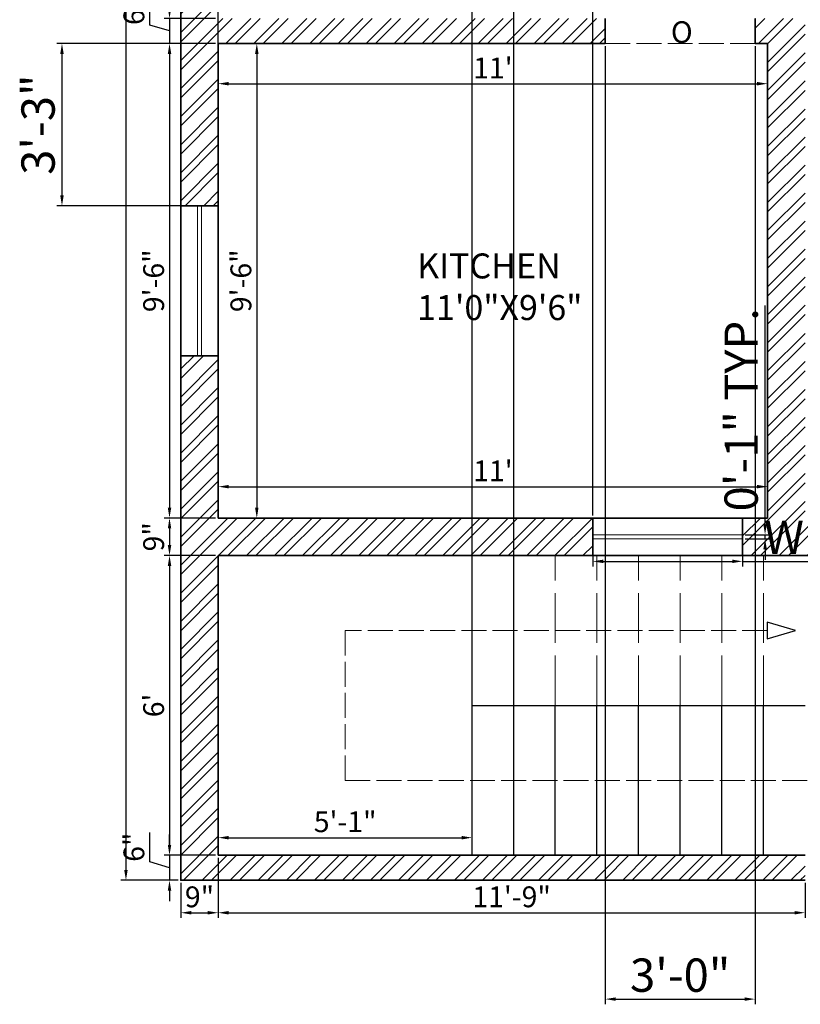
# Model space of a CAD drawing. Units: inches. Extents: x 3595 to 4516, y 2363 to 2965.
# Tile 1 of 12: x 3601 to 3789, y 2369 to 2606. Entities that reach past the tile are written whole.
import ezdxf

# ---------------------------------------------------------------- set-up
doc = ezdxf.new("R2010")
doc.units = ezdxf.units.IN
doc.linetypes.add('ACAD_ISO02W100', pattern=[15, 12, -3])
for name, color, linetype, lineweight in [('A-ANNO-DIMS', 2, 'Continuous', 18), ('A-ANNO-TEXT', 7, 'Continuous', 25), ('A-AREA-IDEN', 7, 'Continuous', 18), ('A-FLOR-STRS', 7, 'Continuous', 25), ('A-FLOR-STRS-OVHD', 7, 'ACAD_ISO02W100', 18), ('A-GLAZ', 4, 'Continuous', 18), ('A-WALL', 7, 'Continuous', 35), ('A-WALL-OVHD', 7, 'ACAD_ISO02W100', 18)]:
    doc.layers.add(name, color=color, linetype=linetype, lineweight=lineweight)
doc.layers.add('A-WALL-PATT', color=251, linetype='Continuous', lineweight=13, true_color=0x636466)
doc.styles.get("Standard").update_dxf_attribs({"font": 'arial.ttf'})
doc.dimstyles.new('ISO-25', dxfattribs={"dimtxt": 8, "dimasz": 2.5, "dimexe": 1.25, "dimexo": 0.625, "dimtad": 1, "dimdec": 1, "dimlunit": 3, "dimtxsty": 'Standard', "dimcen": 2.5, "dimadec": 0, "dimazin": 0, "dimtfac": 1, "dimtdec": 1, "dimtmove": 0, "dimatfit": 3, "dimfxl": 1, "dimarcsym": 0})

# ---------------------------------------------------------------- blocks, each defined once
blk = doc.blocks.new('*D48')
at = {"layer": 'A-ANNO-DIMS', "color": 0, "lineweight": -2, "transparency": 16777216}
for p, q in [((3649.52, 2600.04), (3659.41, 2600.04)), ((3658.16, 2597.54), (3658.16, 2488.54)), ((3649.52, 2486.04), (3659.41, 2486.04))]:
    blk.add_line(p, q, dxfattribs=at)
at = {"layer": 'A-ANNO-DIMS', "color": 0, "transparency": 16777216}
for points in [[(3657.74, 2597.54), (3658.57, 2597.54), (3658.16, 2600.04)], [(3657.74, 2488.54), (3658.57, 2488.54), (3658.16, 2486.04)]]:
    blk.add_solid(points, dxfattribs=at)
at = {"layer": 'Defpoints', "color": 0, "transparency": 16777216}
for p in [(3648.89, 2600.04), (3648.89, 2486.04), (3658.16, 2486.04)]:
    blk.add_point(p, dxfattribs=at)
at = {"layer": 'A-ANNO-DIMS', "color": 0, "transparency": 16777216, "insert": (3654.98, 2543.04), "char_height": 5, "attachment_point": 5, "rotation": 90}
blk.add_mtext('9\'-6"', dxfattribs=at)
blk = doc.blocks.new('*D49')
at = {"layer": 'A-ANNO-DIMS', "color": 0, "lineweight": -2, "transparency": 16777216}
for p, q in [((3648.89, 2599.42), (3648.89, 2589.13)), ((3780.89, 2599.42), (3780.89, 2589.13)), ((3651.39, 2590.38), (3778.39, 2590.38))]:
    blk.add_line(p, q, dxfattribs=at)
at = {"layer": 'A-ANNO-DIMS', "color": 0, "transparency": 16777216}
for points in [[(3651.39, 2590.79), (3651.39, 2589.96), (3648.89, 2590.38)], [(3778.39, 2590.79), (3778.39, 2589.96), (3780.89, 2590.38)]]:
    blk.add_solid(points, dxfattribs=at)
at = {"layer": 'Defpoints', "color": 0, "transparency": 16777216}
for p in [(3648.89, 2600.04), (3780.89, 2600.04), (3780.89, 2590.38)]:
    blk.add_point(p, dxfattribs=at)
at = {"layer": 'A-ANNO-DIMS', "color": 0, "transparency": 16777216, "insert": (3714.89, 2593.51), "char_height": 5, "attachment_point": 5}
blk.add_mtext("11'", dxfattribs=at)
blk = doc.blocks.new('*D55')
at = {"layer": 'A-ANNO-DIMS', "color": 0, "lineweight": -2, "transparency": 16777216}
for p, q in [((3648.89, 2486.67), (3648.89, 2494.83)), ((3651.39, 2493.58), (3778.39, 2493.58)), ((3780.89, 2486.67), (3780.89, 2494.83))]:
    blk.add_line(p, q, dxfattribs=at)
at = {"layer": 'A-ANNO-DIMS', "color": 0, "transparency": 16777216}
for points in [[(3651.39, 2494), (3651.39, 2493.17), (3648.89, 2493.58)], [(3778.39, 2494), (3778.39, 2493.17), (3780.89, 2493.58)]]:
    blk.add_solid(points, dxfattribs=at)
at = {"layer": 'Defpoints', "color": 0, "transparency": 16777216}
for p in [(3780.89, 2493.58), (3648.89, 2486.04), (3780.89, 2486.04)]:
    blk.add_point(p, dxfattribs=at)
at = {"layer": 'A-ANNO-DIMS', "color": 0, "transparency": 16777216, "insert": (3714.89, 2496.72), "char_height": 5, "attachment_point": 5}
blk.add_mtext("11'", dxfattribs=at)
blk = doc.blocks.new('*D56')
at = {"layer": 'A-ANNO-DIMS', "color": 0, "lineweight": -2, "transparency": 16777216}
for p, q in [((3648.89, 2405.67), (3648.89, 2410.52)), ((3709.89, 2405.67), (3709.89, 2410.52)), ((3651.39, 2409.27), (3707.39, 2409.27))]:
    blk.add_line(p, q, dxfattribs=at)
at = {"layer": 'A-ANNO-DIMS', "color": 0, "transparency": 16777216}
for points in [[(3651.39, 2409.69), (3651.39, 2408.85), (3648.89, 2409.27)], [(3707.39, 2409.69), (3707.39, 2408.85), (3709.89, 2409.27)]]:
    blk.add_solid(points, dxfattribs=at)
at = {"layer": 'Defpoints', "color": 0, "transparency": 16777216}
for p in [(3709.89, 2409.27), (3648.89, 2405.04), (3709.89, 2405.04)]:
    blk.add_point(p, dxfattribs=at)
at = {"layer": 'A-ANNO-DIMS', "color": 0, "transparency": 16777216, "insert": (3679.39, 2412.45), "char_height": 5, "attachment_point": 5}
blk.add_mtext('5\'-1"', dxfattribs=at)
blk = doc.blocks.new('*D73')
at = {"layer": 'A-ANNO-DIMS', "color": 0, "lineweight": -2, "transparency": 16777216}
for p, q in [((3632.44, 2604.47), (3632.44, 2611.49)), ((3637.18, 2608.54), (3637.18, 2611.04)), ((3637.18, 2603.04), (3632.44, 2604.47)), ((3648.27, 2606.04), (3635.93, 2606.04)), ((3637.18, 2606.04), (3637.18, 2600.04)), ((3637.18, 2606.04), (3637.18, 2600.04)), ((3648.27, 2600.04), (3635.93, 2600.04)), ((3637.18, 2597.54), (3637.18, 2595.04))]:
    blk.add_line(p, q, dxfattribs=at)
at = {"layer": 'A-ANNO-DIMS', "color": 0, "transparency": 16777216}
for points in [[(3636.77, 2608.54), (3637.6, 2608.54), (3637.18, 2606.04)], [(3636.77, 2597.54), (3637.6, 2597.54), (3637.18, 2600.04)]]:
    blk.add_solid(points, dxfattribs=at)
at = {"layer": 'Defpoints', "color": 0, "transparency": 16777216}
for p in [(3648.89, 2606.04), (3637.18, 2600.04), (3648.89, 2600.04)]:
    blk.add_point(p, dxfattribs=at)
at = {"layer": 'A-ANNO-DIMS', "color": 0, "transparency": 16777216, "insert": (3629.27, 2607.98), "char_height": 5, "attachment_point": 5, "rotation": 90}
blk.add_mtext('6"', dxfattribs=at)
blk = doc.blocks.new('*D74')
at = {"layer": 'A-ANNO-DIMS', "color": 0, "lineweight": -2, "transparency": 16777216}
for p, q in [((3648.27, 2600.04), (3635.93, 2600.04)), ((3637.18, 2597.54), (3637.18, 2488.54)), ((3648.27, 2486.04), (3635.93, 2486.04))]:
    blk.add_line(p, q, dxfattribs=at)
at = {"layer": 'A-ANNO-DIMS', "color": 0, "transparency": 16777216}
for points in [[(3636.77, 2597.54), (3637.6, 2597.54), (3637.18, 2600.04)], [(3636.77, 2488.54), (3637.6, 2488.54), (3637.18, 2486.04)]]:
    blk.add_solid(points, dxfattribs=at)
at = {"layer": 'Defpoints', "color": 0, "transparency": 16777216}
for p in [(3648.89, 2600.04), (3637.18, 2486.04), (3648.89, 2486.04)]:
    blk.add_point(p, dxfattribs=at)
at = {"layer": 'A-ANNO-DIMS', "color": 0, "transparency": 16777216, "insert": (3634.01, 2543.04), "char_height": 5, "attachment_point": 5, "rotation": 90}
blk.add_mtext('9\'-6"', dxfattribs=at)
blk = doc.blocks.new('*D75')
at = {"layer": 'A-ANNO-DIMS', "color": 0, "lineweight": -2, "transparency": 16777216}
for p, q in [((3648.27, 2486.04), (3635.93, 2486.04)), ((3637.18, 2483.54), (3637.18, 2479.54)), ((3648.27, 2477.04), (3635.93, 2477.04))]:
    blk.add_line(p, q, dxfattribs=at)
at = {"layer": 'A-ANNO-DIMS', "color": 0, "transparency": 16777216}
for points in [[(3636.77, 2483.54), (3637.6, 2483.54), (3637.18, 2486.04)], [(3636.77, 2479.54), (3637.6, 2479.54), (3637.18, 2477.04)]]:
    blk.add_solid(points, dxfattribs=at)
at = {"layer": 'Defpoints', "color": 0, "transparency": 16777216}
for p in [(3648.89, 2486.04), (3637.18, 2477.04), (3648.89, 2477.04)]:
    blk.add_point(p, dxfattribs=at)
at = {"layer": 'A-ANNO-DIMS', "color": 0, "transparency": 16777216, "insert": (3634.01, 2481.54), "char_height": 5, "attachment_point": 5, "rotation": 90}
blk.add_mtext('9"', dxfattribs=at)
blk = doc.blocks.new('*D76')
at = {"layer": 'A-ANNO-DIMS', "color": 0, "lineweight": -2, "transparency": 16777216}
for p, q in [((3648.27, 2477.04), (3635.93, 2477.04)), ((3637.18, 2474.54), (3637.18, 2407.54)), ((3648.27, 2405.04), (3635.93, 2405.04))]:
    blk.add_line(p, q, dxfattribs=at)
at = {"layer": 'A-ANNO-DIMS', "color": 0, "transparency": 16777216}
for points in [[(3636.77, 2474.54), (3637.6, 2474.54), (3637.18, 2477.04)], [(3636.77, 2407.54), (3637.6, 2407.54), (3637.18, 2405.04)]]:
    blk.add_solid(points, dxfattribs=at)
at = {"layer": 'Defpoints', "color": 0, "transparency": 16777216}
for p in [(3648.89, 2477.04), (3637.18, 2405.04), (3648.89, 2405.04)]:
    blk.add_point(p, dxfattribs=at)
at = {"layer": 'A-ANNO-DIMS', "color": 0, "transparency": 16777216, "insert": (3634.01, 2441.04), "char_height": 5, "attachment_point": 5, "rotation": 90}
blk.add_mtext("6'", dxfattribs=at)
blk = doc.blocks.new('*D77')
at = {"layer": 'A-ANNO-DIMS', "color": 0, "lineweight": -2, "transparency": 16777216}
for p, q in [((3632.44, 2403.47), (3632.44, 2410.49)), ((3637.18, 2407.54), (3637.18, 2410.04)), ((3637.18, 2402.04), (3632.44, 2403.47)), ((3648.27, 2405.04), (3635.93, 2405.04)), ((3637.18, 2405.04), (3637.18, 2399.04)), ((3637.18, 2405.04), (3637.18, 2399.04)), ((3639.27, 2399.04), (3635.93, 2399.04)), ((3637.18, 2396.54), (3637.18, 2394.04))]:
    blk.add_line(p, q, dxfattribs=at)
at = {"layer": 'A-ANNO-DIMS', "color": 0, "transparency": 16777216}
for points in [[(3636.77, 2407.54), (3637.6, 2407.54), (3637.18, 2405.04)], [(3636.77, 2396.54), (3637.6, 2396.54), (3637.18, 2399.04)]]:
    blk.add_solid(points, dxfattribs=at)
at = {"layer": 'Defpoints', "color": 0, "transparency": 16777216}
for p in [(3648.89, 2405.04), (3637.18, 2399.04), (3639.89, 2399.04)]:
    blk.add_point(p, dxfattribs=at)
at = {"layer": 'A-ANNO-DIMS', "color": 0, "transparency": 16777216, "insert": (3629.27, 2406.98), "char_height": 5, "attachment_point": 5, "rotation": 90}
blk.add_mtext('6"', dxfattribs=at)
blk = doc.blocks.new('*D78')
at = {"layer": 'A-ANNO-DIMS', "color": 0, "lineweight": -2, "transparency": 16777216}
for p, q in [((3648.89, 2404.42), (3648.89, 2389.99)), ((3639.89, 2398.42), (3639.89, 2389.99)), ((3642.39, 2391.24), (3646.39, 2391.24))]:
    blk.add_line(p, q, dxfattribs=at)
at = {"layer": 'A-ANNO-DIMS', "color": 0, "transparency": 16777216}
for points in [[(3642.39, 2391.65), (3642.39, 2390.82), (3639.89, 2391.24)], [(3646.39, 2391.65), (3646.39, 2390.82), (3648.89, 2391.24)]]:
    blk.add_solid(points, dxfattribs=at)
at = {"layer": 'Defpoints', "color": 0, "transparency": 16777216}
for p in [(3648.89, 2405.04), (3639.89, 2399.04), (3648.89, 2391.24)]:
    blk.add_point(p, dxfattribs=at)
at = {"layer": 'A-ANNO-DIMS', "color": 0, "transparency": 16777216, "insert": (3644.39, 2394.41), "char_height": 5, "attachment_point": 5}
blk.add_mtext('9"', dxfattribs=at)
blk = doc.blocks.new('*D79')
at = {"layer": 'A-ANNO-DIMS', "color": 0, "lineweight": -2, "transparency": 16777216}
for p, q in [((3648.89, 2404.42), (3648.89, 2389.99)), ((3789.89, 2398.42), (3789.89, 2389.99)), ((3651.39, 2391.24), (3787.39, 2391.24))]:
    blk.add_line(p, q, dxfattribs=at)
at = {"layer": 'A-ANNO-DIMS', "color": 0, "transparency": 16777216}
for points in [[(3651.39, 2391.65), (3651.39, 2390.82), (3648.89, 2391.24)], [(3787.39, 2391.65), (3787.39, 2390.82), (3789.89, 2391.24)]]:
    blk.add_solid(points, dxfattribs=at)
at = {"layer": 'Defpoints', "color": 0, "transparency": 16777216}
for p in [(3648.89, 2405.04), (3789.89, 2399.04), (3789.89, 2391.24)]:
    blk.add_point(p, dxfattribs=at)
at = {"layer": 'A-ANNO-DIMS', "color": 0, "transparency": 16777216, "insert": (3719.39, 2394.41), "char_height": 5, "attachment_point": 5}
blk.add_mtext('11\'-9"', dxfattribs=at)
blk = doc.blocks.new('*D90')
at = {"layer": 'A-ANNO-DIMS', "color": 0, "lineweight": -2, "transparency": 16777216}
for p, q in [((3639.27, 2903.04), (3625.46, 2903.04)), ((3626.71, 2900.54), (3626.71, 2401.54)), ((3639.27, 2399.04), (3625.46, 2399.04))]:
    blk.add_line(p, q, dxfattribs=at)
at = {"layer": 'A-ANNO-DIMS', "color": 0, "transparency": 16777216}
for points in [[(3626.3, 2900.54), (3627.13, 2900.54), (3626.71, 2903.04)], [(3626.3, 2401.54), (3627.13, 2401.54), (3626.71, 2399.04)]]:
    blk.add_solid(points, dxfattribs=at)
at = {"layer": 'Defpoints', "color": 0, "transparency": 16777216}
for p in [(3639.89, 2903.04), (3626.71, 2399.04), (3639.89, 2399.04)]:
    blk.add_point(p, dxfattribs=at)
at = {"layer": 'A-ANNO-DIMS', "color": 0, "transparency": 16777216, "insert": (3623.58, 2651.04), "char_height": 5, "attachment_point": 5, "rotation": 90}
blk.add_mtext("42'", dxfattribs=at)
blk = doc.blocks.new('WIN-GLAZING-36IN')
for p, q in [((0, 1), (36, 1)), ((0, 0), (36, 0))]:
    blk.add_line(p, q)
blk = doc.blocks.new('*D101')
at = {"layer": 'A-ANNO-DIMS', "color": 0, "lineweight": -2, "transparency": 16777216}
for p, q in [((3738.89, 2480.42), (3738.89, 2474.39)), ((3774.89, 2480.42), (3774.89, 2474.39)), ((3741.39, 2475.64), (3772.39, 2475.64)), ((3774.89, 2475.64), (3879.88, 2475.64))]:
    blk.add_line(p, q, dxfattribs=at)
at = {"layer": 'A-ANNO-DIMS', "color": 0, "transparency": 16777216}
for points in [[(3741.39, 2476.06), (3741.39, 2475.23), (3738.89, 2475.64)], [(3772.39, 2476.06), (3772.39, 2475.23), (3774.89, 2475.64)]]:
    blk.add_solid(points, dxfattribs=at)
at = {"layer": 'Defpoints', "color": 0, "transparency": 16777216}
for p in [(3738.89, 2481.04), (3774.89, 2481.04), (3774.89, 2475.64)]:
    blk.add_point(p, dxfattribs=at)
at = {"layer": 'A-ANNO-DIMS', "color": 0, "transparency": 16777216, "insert": (3828.63, 2480.41), "char_height": 8, "attachment_point": 5}
blk.add_mtext('WINDOW 3\'-0" TYP.', dxfattribs=at)
blk = doc.blocks.new('*D102')
at = {"layer": 'A-ANNO-DIMS', "color": 0, "lineweight": -2, "transparency": 16777216}
for p, q in [((3780.29, 2484.54), (3780.29, 2537.06)), ((3775.52, 2482.04), (3781.54, 2482.04)), ((3775.52, 2481.04), (3781.54, 2481.04)), ((3780.29, 2481.04), (3780.29, 2482.04)), ((3780.29, 2478.54), (3780.29, 2476.04))]:
    blk.add_line(p, q, dxfattribs=at)
at = {"layer": 'A-ANNO-DIMS', "color": 0, "transparency": 16777216}
for points in [[(3779.88, 2484.54), (3780.71, 2484.54), (3780.29, 2482.04)], [(3779.88, 2478.54), (3780.71, 2478.54), (3780.29, 2481.04)]]:
    blk.add_solid(points, dxfattribs=at)
at = {"layer": 'Defpoints', "color": 0, "transparency": 16777216}
for p in [(3774.89, 2482.04), (3774.89, 2481.04), (3780.29, 2482.04)]:
    blk.add_point(p, dxfattribs=at)
at = {"layer": 'A-ANNO-DIMS', "color": 0, "transparency": 16777216, "insert": (3775.58, 2512.05), "char_height": 8, "attachment_point": 5, "rotation": 90}
blk.add_mtext('0\'-1" TYP.', dxfattribs=at)
blk = doc.blocks.new('*D152')
at = {"layer": 'A-ANNO-DIMS', "color": 0, "lineweight": -2, "transparency": 16777216}
for p, q in [((3648.27, 2600.04), (3610.09, 2600.04)), ((3611.34, 2597.54), (3611.34, 2563.54)), ((3648.27, 2561.04), (3610.09, 2561.04))]:
    blk.add_line(p, q, dxfattribs=at)
at = {"layer": 'A-ANNO-DIMS', "color": 0, "transparency": 16777216}
for points in [[(3610.93, 2597.54), (3611.76, 2597.54), (3611.34, 2600.04)], [(3610.93, 2563.54), (3611.76, 2563.54), (3611.34, 2561.04)]]:
    blk.add_solid(points, dxfattribs=at)
at = {"layer": 'Defpoints', "color": 0, "transparency": 16777216}
for p in [(3648.89, 2600.04), (3611.34, 2561.04), (3648.89, 2561.04)]:
    blk.add_point(p, dxfattribs=at)
at = {"layer": 'A-ANNO-DIMS', "color": 0, "transparency": 16777216, "insert": (3606.63, 2580.54), "char_height": 8, "attachment_point": 5, "rotation": 90}
blk.add_mtext('3\'-3"', dxfattribs=at)
blk = doc.blocks.new('*D156')
at = {"layer": 'A-ANNO-DIMS', "color": 0, "lineweight": -2, "transparency": 16777216}
for p, q in [((3648.89, 2486.67), (3648.89, 2932.84)), ((3738.89, 2486.67), (3738.89, 2932.84)), ((3651.39, 2931.59), (3736.39, 2931.59))]:
    blk.add_line(p, q, dxfattribs=at)
at = {"layer": 'A-ANNO-DIMS', "color": 0, "transparency": 16777216}
for points in [[(3651.39, 2932.01), (3651.39, 2931.18), (3648.89, 2931.59)], [(3736.39, 2932.01), (3736.39, 2931.18), (3738.89, 2931.59)]]:
    blk.add_solid(points, dxfattribs=at)
at = {"layer": 'Defpoints', "color": 0, "transparency": 16777216}
for p in [(3738.89, 2931.59), (3648.89, 2486.04), (3738.89, 2486.04)]:
    blk.add_point(p, dxfattribs=at)
at = {"layer": 'A-ANNO-DIMS', "color": 0, "transparency": 16777216, "insert": (3693.89, 2936.3), "char_height": 8, "attachment_point": 5}
blk.add_mtext('7\'-6"', dxfattribs=at)
blk = doc.blocks.new('*D158')
at = {"layer": 'A-ANNO-DIMS', "color": 0, "lineweight": -2, "transparency": 16777216}
for p, q in [((3741.89, 2599.42), (3741.89, 2369.24)), ((3777.89, 2599.42), (3777.89, 2369.24)), ((3744.39, 2370.49), (3775.39, 2370.49))]:
    blk.add_line(p, q, dxfattribs=at)
at = {"layer": 'A-ANNO-DIMS', "color": 0, "transparency": 16777216}
for points in [[(3744.39, 2370.91), (3744.39, 2370.08), (3741.89, 2370.49)], [(3775.39, 2370.91), (3775.39, 2370.08), (3777.89, 2370.49)]]:
    blk.add_solid(points, dxfattribs=at)
at = {"layer": 'Defpoints', "color": 0, "transparency": 16777216}
for p in [(3741.89, 2600.04), (3777.89, 2600.04), (3777.89, 2370.49)]:
    blk.add_point(p, dxfattribs=at)
at = {"layer": 'A-ANNO-DIMS', "color": 0, "transparency": 16777216, "insert": (3759.89, 2375.21), "char_height": 8, "attachment_point": 5}
blk.add_mtext('3\'-0"', dxfattribs=at)
blk = doc.blocks.new('*D159')
at = {"layer": 'A-ANNO-DIMS', "color": 0, "lineweight": -2, "transparency": 16777216}
for p, q in [((3709.89, 2405.67), (3709.89, 2932.84)), ((3719.89, 2405.67), (3719.89, 2932.84)), ((3712.39, 2931.59), (3717.39, 2931.59)), ((3719.89, 2931.59), (3751.12, 2931.59))]:
    blk.add_line(p, q, dxfattribs=at)
at = {"layer": 'A-ANNO-DIMS', "color": 0, "transparency": 16777216}
for points in [[(3712.39, 2932.01), (3712.39, 2931.18), (3709.89, 2931.59)], [(3717.39, 2932.01), (3717.39, 2931.18), (3719.89, 2931.59)]]:
    blk.add_solid(points, dxfattribs=at)
at = {"layer": 'Defpoints', "color": 0, "transparency": 16777216}
for p in [(3719.89, 2931.59), (3709.89, 2405.04), (3719.89, 2405.04)]:
    blk.add_point(p, dxfattribs=at)
at = {"layer": 'A-ANNO-DIMS', "color": 0, "transparency": 16777216, "insert": (3736.76, 2936.3), "char_height": 8, "attachment_point": 5}
blk.add_mtext('0\'-10"', dxfattribs=at)

msp = doc.modelspace()

# ---------------------------------------------------------------- hatches: boundary and pattern name
at = {"layer": 'A-WALL-PATT'}
h = msp.add_hatch(dxfattribs=at)
h.set_pattern_fill('ANSI32', color=256, scale=0.5)
h.paths.add_polyline_path([(3648.89, 2894.04), (3726.89, 2894.04), (3726.89, 2903.04), (3639.89, 2903.04), (3639.89, 2756.04), (3648.89, 2756.04)])
h.paths.add_polyline_path([(3800.39, 2903.04), (3774.89, 2903.04), (3774.89, 2894.04), (3780.89, 2894.04), (3780.89, 2792.04), (3789.89, 2792.04), (3789.89, 2894.04), (3800.39, 2894.04)])
h.paths.add_polyline_path([(3882.89, 2903.04), (3836.39, 2903.04), (3836.39, 2894.04), (3846.89, 2894.04), (3846.89, 2798.04), (3819.89, 2798.04), (3819.89, 2792.04), (3846.89, 2792.04), (3846.89, 2756.04), (3780.89, 2756.04), (3780.89, 2702.04), (3777.89, 2702.04), (3777.89, 2693.04), (3800.39, 2693.04), (3800.39, 2702.04), (3789.89, 2702.04), (3789.89, 2750.04), (3846.89, 2750.04), (3846.89, 2702.04), (3836.39, 2702.04), (3836.39, 2693.04), (3951.89, 2693.04), (3951.89, 2702.04), (3852.89, 2702.04), (3852.89, 2840.04), (3954.89, 2840.04), (3954.89, 2846.04), (3852.89, 2846.04), (3852.89, 2894.04), (3882.89, 2894.04)])
h.paths.add_polyline_path([(3999.89, 2903.04), (3918.89, 2903.04), (3918.89, 2894.04), (3948.89, 2894.04), (3948.89, 2876.04), (3954.89, 2876.04), (3954.89, 2894.04), (3990.89, 2894.04), (3990.89, 2795.04), (3999.89, 2795.04)])
h.paths.add_polyline_path([(3741.89, 2702.04), (3648.89, 2702.04), (3648.89, 2708.04), (3639.89, 2708.04), (3639.89, 2673.54), (3648.89, 2673.54), (3648.89, 2693.04), (3741.89, 2693.04)])
h.paths.add_polyline_path([(3648.89, 2600.04), (3741.89, 2600.04), (3741.89, 2606.04), (3648.89, 2606.04), (3648.89, 2625.54), (3639.89, 2625.54), (3639.89, 2561.04), (3648.89, 2561.04)])
h.paths.add_polyline_path([(3648.89, 2525.04), (3639.89, 2525.04), (3639.89, 2399.04), (3789.89, 2399.04), (3789.89, 2405.04), (3648.89, 2405.04), (3648.89, 2477.04), (3738.89, 2477.04), (3738.89, 2486.04), (3648.89, 2486.04)])
h.paths.add_polyline_path([(3789.89, 2606.04), (3777.89, 2606.04), (3777.89, 2600.04), (3780.89, 2600.04), (3780.89, 2486.04), (3774.89, 2486.04), (3774.89, 2477.04), (3831.89, 2477.04), (3831.89, 2486.04), (3789.89, 2486.04)])
h.paths.add_polyline_path([(3939.89, 2486.04), (3897.89, 2486.04), (3897.89, 2477.04), (3939.89, 2477.04)])
h.paths.add_polyline_path([(3999.89, 2511.54), (3990.89, 2511.54), (3990.89, 2486.04), (3987.89, 2486.04), (3987.89, 2477.04), (3999.89, 2477.04)])
h.paths.add_polyline_path([(3999.89, 2607.54), (3990.89, 2607.54), (3990.89, 2571.54), (3999.89, 2571.54)])
h.paths.add_polyline_path([(3999.89, 2747.04), (3990.89, 2747.04), (3990.89, 2702.04), (3987.89, 2702.04), (3987.89, 2693.04), (3990.89, 2693.04), (3990.89, 2667.54), (3999.89, 2667.54)])

# ---------------------------------------------------------------- linework, layer by layer
at = {"layer": 'A-FLOR-STRS'}
for p, q in [((3709.89, 2405.04), (3709.89, 2441.04)), ((3709.89, 2441.04), (3789.89, 2441.04)), ((3719.89, 2405.04), (3719.89, 2441.04)), ((3729.89, 2405.04), (3729.89, 2441.04)), ((3739.89, 2405.04), (3739.89, 2441.04)), ((3749.89, 2405.04), (3749.89, 2441.04)), ((3759.89, 2405.04), (3759.89, 2441.04)), ((3769.89, 2405.04), (3769.89, 2441.04)), ((3779.89, 2405.04), (3779.89, 2441.04))]:
    msp.add_line(p, q, dxfattribs=at)
msp.add_lwpolyline([(3787.63, 2459.04), (3780.82, 2461.04), (3780.82, 2457.04)], close=True, dxfattribs=at)
at = {"layer": 'A-FLOR-STRS-OVHD'}
for p, q in [((3709.89, 2441.04), (3709.89, 2477.04)), ((3719.89, 2441.04), (3719.89, 2477.04)), ((3729.89, 2441.04), (3729.89, 2477.04)), ((3739.89, 2441.04), (3739.89, 2477.04)), ((3749.89, 2441.04), (3749.89, 2477.04)), ((3759.89, 2441.04), (3759.89, 2477.04)), ((3769.89, 2441.04), (3769.89, 2477.04)), ((3779.89, 2441.04), (3779.89, 2477.04))]:
    msp.add_line(p, q, dxfattribs=at)
at = {"layer": 'A-FLOR-STRS-OVHD', "ltscale": 0.5}
msp.add_lwpolyline([(3780.82, 2459.04), (3679.39, 2459.04), (3679.39, 2423.04), (3798.62, 2423.04)], dxfattribs=at)
at = {"layer": 'A-WALL'}
for p, q in [((3741.89, 2606.04), (3741.89, 2600.04)), ((3777.89, 2606.04), (3777.89, 2600.04)), ((3648.89, 2600.04), (3741.89, 2600.04)), ((3648.89, 2486.04), (3648.89, 2600.04)), ((3777.89, 2600.04), (3780.89, 2600.04)), ((3780.89, 2486.04), (3780.89, 2600.04)), ((3648.89, 2561.04), (3639.89, 2561.04)), ((3648.89, 2525.04), (3639.89, 2525.04)), ((3648.89, 2486.04), (3780.89, 2486.04)), ((3738.89, 2477.04), (3738.89, 2486.04)), ((3774.89, 2477.04), (3774.89, 2486.04)), ((3648.89, 2405.04), (3648.89, 2477.04)), ((3648.89, 2477.04), (3939.89, 2477.04)), ((3648.89, 2405.04), (3789.89, 2405.04))]:
    msp.add_line(p, q, dxfattribs=at)
msp.add_lwpolyline([(3789.89, 2399.04), (3639.89, 2399.04), (3639.89, 2903.04), (3999.89, 2903.04), (3999.89, 2477.04)], dxfattribs=at)
at = {"layer": 'A-WALL-OVHD', "ltscale": 0.5}
msp.add_line((3741.89, 2600.04), (3777.89, 2600.04), dxfattribs=at)

# ---------------------------------------------------------------- block references
at = {"layer": 'A-GLAZ', "rotation": 269.9999999999999}
msp.add_blockref('WIN-GLAZING-36IN', (3643.89, 2561.04), dxfattribs=at)
at = {"layer": 'A-GLAZ'}
msp.add_blockref('WIN-GLAZING-36IN', (3738.89, 2481.04), dxfattribs=at)

# ---------------------------------------------------------------- texts
at = {"layer": 'A-ANNO-TEXT'}
msp.add_text('O', height=5.18, dxfattribs=at).set_placement((3757.66, 2600.18))
at = {"layer": 'A-AREA-IDEN', "insert": (3696.68, 2549.6), "char_height": 6, "attachment_point": 1}
msp.add_mtext_dynamic_manual_height_columns('{\\fTimes New Roman|b0|i0|c0|p18;KITCHEN\\P11\'0"X9\'6"}', width=67.3508, gutter_width=12.5, heights=[0], dxfattribs=at)

# ---------------------------------------------------------------- dimensions: what is measured, and where the dimension line sits
at = {"layer": 'A-ANNO-DIMS'}
for base, p1, p2, override, picture, middle in [((3738.89, 2931.59), (3648.89, 2486.04), (3738.89, 2486.04), {"dimdec": 1, "dimlfac": 1, "dimrnd": 0, "dimzin": 1, "dimdsep": 46, "dimlunit": 4, "dimfrac": 2}, '*D156', (3693.89, 2936.3)), ((3719.89, 2931.59), (3709.89, 2405.04), (3719.89, 2405.04), {"dimdec": 1, "dimlfac": 1, "dimrnd": 0, "dimzin": 1, "dimdsep": 46, "dimlunit": 4, "dimfrac": 2}, '*D159', (3736.76, 2936.3)), ((3780.89, 2590.38), (3648.89, 2600.04), (3780.89, 2600.04), {"dimtxt": 5, "dimclrd": 0, "dimclre": 0, "dimclrt": 0}, '*D49', (3714.89, 2593.51)), ((3777.89, 2370.49), (3741.89, 2600.04), (3777.89, 2600.04), {"dimdec": 1, "dimlfac": 1, "dimrnd": 0, "dimzin": 1, "dimdsep": 46, "dimlunit": 4, "dimfrac": 2}, '*D158', (3759.89, 2375.21)), ((3780.89, 2493.58), (3648.89, 2486.04), (3780.89, 2486.04), {"dimtxt": 5, "dimclrd": 0, "dimclre": 0, "dimclrt": 0}, '*D55', (3714.89, 2496.72)), ((3709.89, 2409.27), (3648.89, 2405.04), (3709.89, 2405.04), {"dimtxt": 5, "dimclrd": 0, "dimclre": 0, "dimclrt": 0}, '*D56', (3679.39, 2412.45)), ((3648.89, 2391.24), (3639.89, 2399.04), (3648.89, 2405.04), {"dimtxt": 5, "dimclrd": 0, "dimclre": 0, "dimclrt": 0}, '*D78', (3644.39, 2394.41)), ((3789.89, 2391.24), (3648.89, 2405.04), (3789.89, 2399.04), {"dimtxt": 5, "dimclrd": 0, "dimclre": 0, "dimclrt": 0, "dimtmove": 1}, '*D79', (3719.39, 2394.41))]:
    dim = msp.add_linear_dim(base=base, p1=p1, p2=p2, dimstyle='ISO-25', override=override, dxfattribs=at)
    dim.commit()
    dim.dimension.update_dxf_attribs({"geometry": picture, "text_midpoint": middle})
for base, p1, p2, override, picture, middle in [((3626.71, 2399.04), (3639.89, 2903.04), (3639.89, 2399.04), {"dimtxt": 5, "dimclrd": 0, "dimclre": 0, "dimclrt": 0}, '*D90', (3623.58, 2651.04)), ((3637.18, 2600.04), (3648.89, 2606.04), (3648.89, 2600.04), {"dimtxt": 5, "dimclrd": 0, "dimclre": 0, "dimclrt": 0, "dimtmove": 1}, '*D73', (3629.27, 2605.09)), ((3611.34, 2561.04), (3648.89, 2600.04), (3648.89, 2561.04), {"dimdec": 1, "dimlfac": 1, "dimrnd": 0, "dimzin": 1, "dimdsep": 46, "dimlunit": 4, "dimfrac": 2}, '*D152', (3606.63, 2580.54)), ((3637.18, 2486.04), (3648.89, 2600.04), (3648.89, 2486.04), {"dimtxt": 5, "dimclrd": 0, "dimclre": 0, "dimclrt": 0, "dimtmove": 1}, '*D74', (3634.01, 2543.04)), ((3658.16, 2486.04), (3648.89, 2600.04), (3648.89, 2486.04), {"dimtxt": 5, "dimclrd": 0, "dimclre": 0, "dimclrt": 0}, '*D48', (3654.98, 2543.04)), ((3637.18, 2477.04), (3648.89, 2486.04), (3648.89, 2477.04), {"dimtxt": 5, "dimclrd": 0, "dimclre": 0, "dimclrt": 0, "dimtmove": 1}, '*D75', (3634.01, 2481.54)), ((3637.18, 2405.04), (3648.89, 2477.04), (3648.89, 2405.04), {"dimtxt": 5, "dimclrd": 0, "dimclre": 0, "dimclrt": 0, "dimtmove": 1}, '*D76', (3634.01, 2441.04)), ((3637.18, 2399.04), (3648.89, 2405.04), (3639.89, 2399.04), {"dimtxt": 5, "dimclrd": 0, "dimclre": 0, "dimclrt": 0, "dimtmove": 1}, '*D77', (3629.27, 2404.09))]:
    dim = msp.add_linear_dim(base=base, p1=p1, p2=p2, angle=90, dimstyle='ISO-25', override=override, dxfattribs=at)
    dim.commit()
    dim.dimension.update_dxf_attribs({"geometry": picture, "text_midpoint": middle})
dim = msp.add_linear_dim(base=(3780.29, 2482.04), p1=(3774.89, 2481.04), p2=(3774.89, 2482.04), angle=90, text='<> TYP.', dimstyle='ISO-25', override={"dimdec": 1, "dimlfac": 1, "dimrnd": 0, "dimzin": 1, "dimdsep": 46, "dimlunit": 4, "dimfrac": 2}, dxfattribs=at)
dim.commit()
dim.dimension.update_dxf_attribs({"geometry": '*D102', "text_midpoint": (3775.58, 2512.05)})
dim = msp.add_linear_dim(base=(3774.89, 2475.64), p1=(3738.89, 2481.04), p2=(3774.89, 2481.04), text='WINDOW <> TYP.', dimstyle='ISO-25', override={"dimdec": 1, "dimlfac": 1, "dimrnd": 0, "dimzin": 1, "dimdsep": 46, "dimlunit": 4, "dimfrac": 2}, dxfattribs=at)
dim.commit()
dim.dimension.update_dxf_attribs({"geometry": '*D101', "text_midpoint": (3828.63, 2480.41)})

doc.saveas('drawing.dxf')
